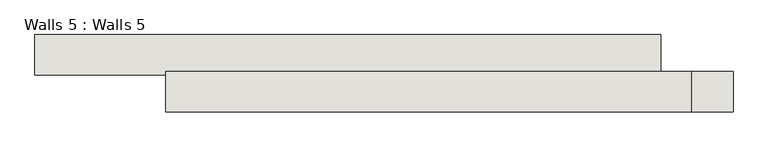
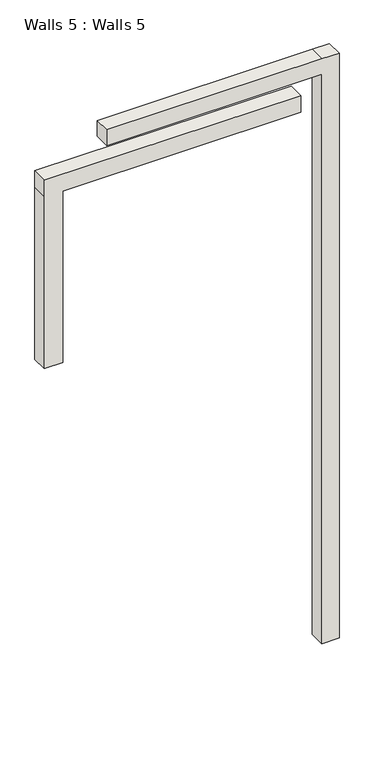
"""IFC4 building model written with IfcOpenShell, lengths in millimetres: wall geometry, Walls 5 : Walls 5."""

from ifc_helpers import new_model, si_unit, frame, origin, place, context, project, spatial, polyline, outline, extrude, source, transform, mapped, element, save


def walls_5_walls_5_fc3546cb(model_context):
    return source(origin(), model_context, "Body", "SweptSolid", [
        extrude(outline(polyline([(7620.0, -6454.7355962), (7620.0, -6115.6864472), (10972.8, -6115.6864472), (10972.8, -1721.4864472), (11303.0, -1721.4864472), (11303.0, -6454.7355962), (10972.8, -6454.7355962), (7620.0, -6454.7355962)])), frame((0.0, 1785.3827135, 0.0), z_axis=(0.0, 1.0, 0.0), x_axis=(0.0, 0.0, 1.0)), (0.0, 0.0, 1.0), 304.8),
        extrude(outline(polyline([(12111.5857686, -1491.2093643), (12111.5857686, -5466.3093643), (11806.7857686, -5466.3093643), (11806.7857686, -1491.2093643), (677.7969121, -1491.2093643), (677.7969121, -1173.7093643), (12111.5857686, -1173.7093643), (12111.5857686, -1491.2093643)])), frame((0.0, 1505.9827135, 0.0), z_axis=(0.0, 1.0, 0.0), x_axis=(0.0, 0.0, 1.0)), (0.0, 0.0, 1.0), 304.8),
    ])


if __name__ == "__main__":
    model = new_model("IFC4")
    model_context = context("Model", 3, world=origin())
    ifc_project = project(units=[si_unit("LENGTHUNIT", "METRE", prefix="MILLI")], contexts=[model_context])
    site = spatial("IfcSite", under=ifc_project)
    building = spatial("IfcBuilding", under=site)
    placement = place(None, origin())
    walls_5_walls_5_shape = walls_5_walls_5_fc3546cb(model_context)
    element("IfcWall", 1, ObjectType="Walls 5 : Walls 5", at=placement, inside=building, context=model_context, shape_type="MappedRepresentation", body=[
        mapped(walls_5_walls_5_shape, transform((0.0, 0.0, 0.0), x_axis=(1.0, 0.0, 0.0), y_axis=(0.0, 1.0, 0.0), z_axis=(0.0, 0.0, 1.0))),
    ])
    save(model, "model.ifc")

# Revit data of these elements
# Element 1 (IfcWall, "Walls 5 : Walls 5")
#   Materials on its faces: "Default Wall"
# Materials
#   "Default Wall": colour RGB 128 128 128, transparency 0
